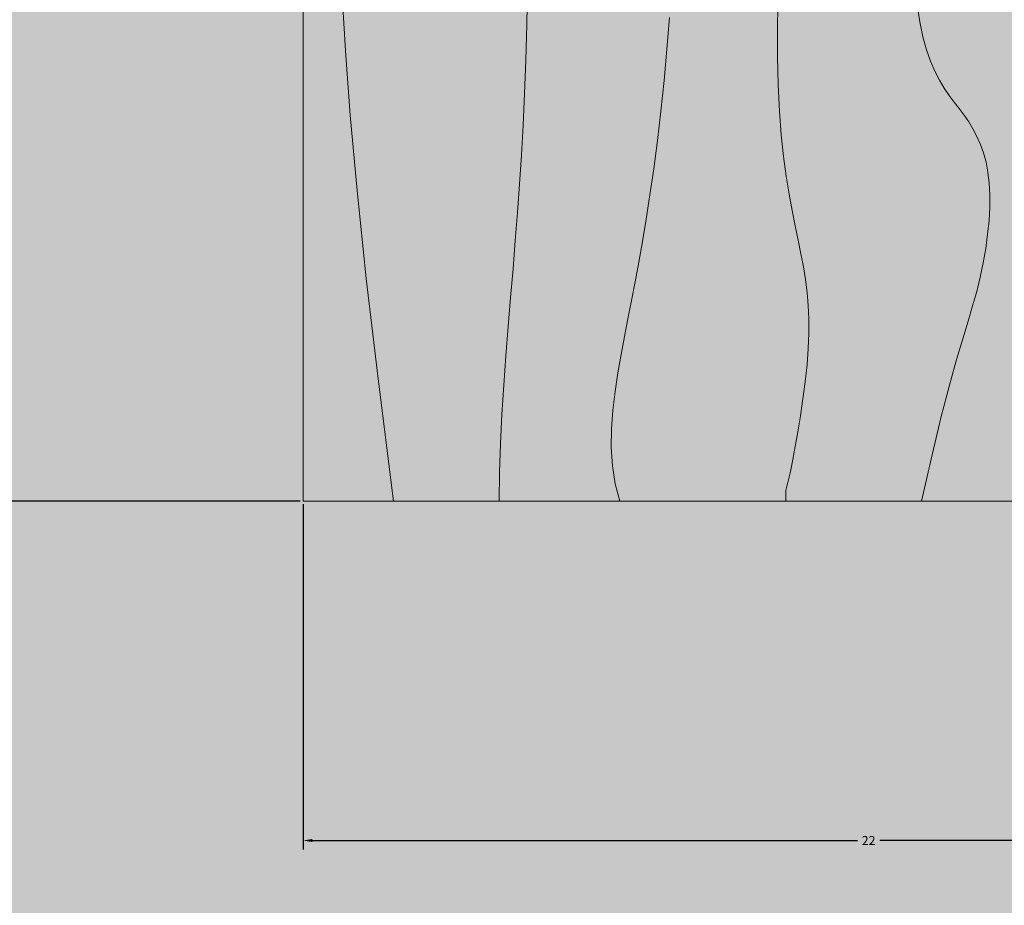
# Model space of a CAD drawing. Units: inches. Extents: x 3024 to 3952, y 1308 to 1863.
# Tile 14 of 29: x 3391.52 to 3411.08, y 1488.75 to 1506.34. Entities that reach past the tile are written whole.
import ezdxf

# ---------------------------------------------------------------- set-up
doc = ezdxf.new("R2010")
doc.units = ezdxf.units.IN
for name, color, linetype, lineweight in [('A-ANNO-DIMS', 2, 'Continuous', 18), ('A-FLOR-TILE-PATT', 7, 'Continuous', 13), ('A-FURN', 8, 'Continuous', 18), ('A-FURN-PATT', 9, 'Continuous', 13)]:
    doc.layers.add(name, color=color, linetype=linetype, lineweight=lineweight)
doc.layers.add('A-FLOR-PATT', color=254, linetype='Continuous', lineweight=13, true_color=0xfeeab9)
doc.styles.get("Standard").update_dxf_attribs({"font": 'arial.ttf'})
doc.dimstyles.get("Standard").update_dxf_attribs({"dimtxt": 0.18, "dimasz": 0.18, "dimexe": 0.18, "dimexo": 0.0625, "dimgap": 0.09, "dimtad": 0, "dimtih": 1, "dimtoh": 1, "dimdec": 4, "dimzin": 0, "dimdsep": 46, "dimtxsty": 'Standard', "dimcen": 0.09, "dimadec": 0, "dimazin": 0, "dimtfac": 1, "dimtdec": 4, "dimtofl": 0, "dimtmove": 0, "dimatfit": 3, "dimfxl": 1, "dimtolj": 1, "dimtzin": 0, "dimarcsym": 0})

# ---------------------------------------------------------------- blocks, each defined once
blk = doc.blocks.new('Table - Rectangular Woodgrain 60 x 30 in.')
for p, q in [((60, -30), (60, 0)), ((0, -30), (60, -30))]:
    blk.add_line(p, q)
for points in [[(46.8439, -13.7104), (47.2906, -13.6417), (47.6858, -13.5604), (48.0333, -13.4667), (48.3375, -13.3608), (48.6042, -13.2448), (48.8396, -13.121), (49.05, -12.9917), (49.2417, -12.8593), (49.4208, -12.7261), (49.5937, -12.5944), (49.7667, -12.4667), (49.9452, -12.3451), (50.1323, -12.2313), (50.3303, -12.1268), (50.5416, -12.0333), (50.7686, -11.9524), (51.0135, -11.8854), (51.2788, -11.8341), (51.5666, -11.8), (51.8785, -11.7843), (52.2116, -11.7865), (52.562, -11.8059), (52.926, -11.8417), (53.2998, -11.8931), (53.6795, -11.9594), (54.0614, -12.0397), (54.4416, -12.1333), (54.8223, -12.2401), (55.2293, -12.3625), (55.6942, -12.5037), (56.2489, -12.6667), (56.9251, -12.8547), (57.7545, -13.0708), (58.7689, -13.3182), (60, -13.6)], [(46.4858, -17.4012), (47.3802, -17.4156), (48.2074, -17.416), (48.9667, -17.4), (49.6583, -17.3662), (50.2872, -17.3167), (50.8595, -17.2547), (51.3812, -17.1833), (51.8584, -17.1057), (52.2971, -17.025), (52.7034, -16.9443), (53.0833, -16.8667), (53.443, -16.7951), (53.789, -16.7313), (54.128, -16.6768), (54.4666, -16.6334), (54.8115, -16.6024), (55.1693, -16.5854), (55.5465, -16.5841), (55.95, -16.6), (56.3828, -16.6337), (56.8346, -16.6823), (57.2915, -16.7418), (57.7396, -16.8084), (58.165, -16.878), (58.5539, -16.9469), (58.8924, -17.0111), (59.1666, -17.0667), (59.3679, -17.1107), (59.5078, -17.1438), (59.6032, -17.1675), (59.6708, -17.1833), (59.7275, -17.193), (59.7901, -17.1979), (59.8753, -17.1998), (60, -17.2)], [(47.1747, -20.2844), (48.0163, -20.3488), (48.8479, -20.425), (49.66, -20.5106), (50.4429, -20.6031), (51.1872, -20.7004), (51.8833, -20.8), (52.5246, -20.8999), (53.1166, -20.9995), (53.6681, -21.0983), (54.1875, -21.1958), (54.6834, -21.2919), (55.1646, -21.3859), (55.6394, -21.4777), (56.1167, -21.5667), (56.6028, -21.6515), (57.0961, -21.7266), (57.5929, -21.7852), (58.0896, -21.8208), (58.5823, -21.8268), (59.0674, -21.7964), (59.5412, -21.723), (60, -21.6)], [(46.3557, -24.0451), (47.3667, -24.0667), (48.309, -24.0947), (49.1928, -24.1287), (50.0284, -24.168), (50.826, -24.2125), (51.5959, -24.2617), (52.3483, -24.3151), (53.0935, -24.3725), (53.8417, -24.4334), (54.6009, -24.497), (55.3699, -24.561), (56.1454, -24.6226), (56.9239, -24.6792), (57.7021, -24.7279), (58.4764, -24.7662), (59.2435, -24.7911), (60, -24.8)], [(46.5843, -28.9641), (48.0579, -28.8816), (49.7666, -28.7542), (51.7629, -28.5721), (54.0989, -28.3255), (56.8272, -28.0048), (60, -27.6)]]:
    blk.add_lwpolyline(points)
blk = doc.blocks.new('*D32')
at = {"layer": 'A-ANNO-DIMS', "color": 0, "lineweight": -2, "transparency": 16777216}
for p, q in [((3397.088, 1541.715), (3390.23, 1541.715)), ((3390.41, 1541.535), (3390.41, 1519.428)), ((3390.41, 1496.958), (3390.41, 1519.065)), ((3397.088, 1496.778), (3390.23, 1496.778))]:
    blk.add_line(p, q, dxfattribs=at)
at = {"layer": 'A-ANNO-DIMS', "color": 0, "transparency": 16777216}
for points in [[(3390.38, 1541.535), (3390.44, 1541.535), (3390.41, 1541.715)], [(3390.38, 1496.958), (3390.44, 1496.958), (3390.41, 1496.778)]]:
    blk.add_solid(points, dxfattribs=at)
at = {"layer": 'Defpoints', "color": 0, "transparency": 16777216}
for p in [(3397.15, 1541.715), (3390.41, 1496.778), (3397.15, 1496.778)]:
    blk.add_point(p, dxfattribs=at)
at = {"layer": 'A-ANNO-DIMS', "color": 0, "transparency": 16777216, "insert": (3390.41, 1519.246), "char_height": 0.18, "attachment_point": 5}
blk.add_mtext('\\A1;TABLE 45', dxfattribs=at)
blk = doc.blocks.new('*D33')
at = {"layer": 'A-ANNO-DIMS', "color": 0, "lineweight": -2, "transparency": 16777216}
for p, q in [((3397.15, 1496.716), (3397.15, 1489.858)), ((3419.618, 1496.716), (3419.618, 1489.858)), ((3397.33, 1490.038), (3408.165, 1490.038)), ((3419.438, 1490.038), (3408.604, 1490.038))]:
    blk.add_line(p, q, dxfattribs=at)
at = {"layer": 'A-ANNO-DIMS', "color": 0, "transparency": 16777216}
for points in [[(3397.33, 1490.068), (3397.33, 1490.008), (3397.15, 1490.038)], [(3419.438, 1490.068), (3419.438, 1490.008), (3419.618, 1490.038)]]:
    blk.add_solid(points, dxfattribs=at)
at = {"layer": 'Defpoints', "color": 0, "transparency": 16777216}
for p in [(3397.15, 1496.778), (3419.618, 1496.778), (3419.618, 1490.038)]:
    blk.add_point(p, dxfattribs=at)
at = {"layer": 'A-ANNO-DIMS', "color": 0, "transparency": 16777216, "insert": (3408.384, 1490.038), "char_height": 0.18, "attachment_point": 5}
blk.add_mtext('\\A1;22', dxfattribs=at)

msp = doc.modelspace()

# ---------------------------------------------------------------- hatches: boundary and pattern name
at = {"layer": 'A-FLOR-PATT', "transparency": 33554528}
h = msp.add_hatch(color=256, dxfattribs=at)
h.dxf.hatch_style = 1
h.paths.add_polyline_path([(3460.764, 1688.6064), (3412.764, 1688.6064), (3412.764, 1694.6064), (3460.764, 1694.6064), (3460.764, 1778.6064), (3406.764, 1778.6064), (3406.764, 1759.9514), (3318.2981, 1759.9514), (3318.2981, 1658.6064), (3322.5356, 1658.6064), (3322.5356, 1652.6064), (3292.764, 1652.6064), (3292.764, 1778.6064), (3106.764, 1778.6064), (3106.764, 1628.6064), (3172.764, 1628.6064), (3172.764, 1532.6064), (3166.764, 1532.6064), (3166.764, 1628.6064), (3106.764, 1628.6064), (3106.764, 1356.8452), (3202.812, 1356.8452), (3202.812, 1354.2534), (3202.812, 1353.8388), (3202.812, 1351.1212), (3202.812, 1347.8452), (3277.764, 1347.8452), (3277.764, 1353.8452), (3277.764, 1356.8452), (3277.764, 1442.6064), (3460.764, 1442.6064)])
h.paths.add_polyline_path([(3216.238, 1527.2064), (3216.238, 1491.2064), (3214.663, 1491.2064), (3214.663, 1491.2409, -0.3966224), (3180.243, 1526.6064), (3163.0285, 1526.6064), (3163.0285, 1531.1064), (3161.716, 1531.1064), (3161.716, 1561.1064), (3163.0285, 1561.1064), (3163.0285, 1531.1064), (3163.0285, 1526.6064), (3180.243, 1526.6064, 0.3966224), (3214.663, 1491.2409), (3214.663, 1527.2064)], flags=16)
h.paths.add_polyline_path([(3227.364, 1649.8972), (3191.364, 1649.8972), (3191.364, 1651.4722), (3227.364, 1651.4722)], flags=16)
h.paths.add_polyline_path([(3323.1172, 1606.7362), (3323.8545, 1606.8514), (3323.8545, 1594.8241), (3323.1172, 1594.9393)], flags=16)
h.paths.add_polyline_path([(3324.2232, 1606.909), (3330.1216, 1607.8307), (3330.1216, 1614.1093), (3339.3495, 1614.1093), (3340.2711, 1620.0078), (3352.4136, 1620.0078), (3353.3353, 1614.1093), (3359.9941, 1614.1093), (3360.9157, 1620.0078), (3373.0582, 1620.0078), (3373.9799, 1614.1093), (3383.2077, 1614.1093), (3383.2077, 1607.8307), (3389.1062, 1606.909), (3389.1062, 1594.7665), (3383.2077, 1593.8449), (3383.2077, 1587.5663), (3373.9799, 1587.5663), (3373.0583, 1581.6678), (3360.9157, 1581.6678), (3359.9941, 1587.5663), (3353.3353, 1587.5663), (3352.4136, 1581.6678), (3340.2711, 1581.6678), (3339.3495, 1587.5663), (3330.1216, 1587.5663), (3330.1216, 1593.8449), (3324.2232, 1594.7665)], flags=16)
h.paths.add_polyline_path([(3236.1584, 1693.1064), (3236.1584, 1723.1064), (3237.4709, 1723.1064), (3237.4709, 1693.1064)], flags=16)
h.paths.add_polyline_path([(3373.2158, 1600.6847), (3373.7965, 1600.7303), (3374.3268, 1600.7874), (3374.8132, 1600.8531), (3375.2621, 1600.9247), (3375.6801, 1600.9991), (3376.0736, 1601.0735), (3376.6855, 1601.19), (3377.366, 1601.3023), (3378.0667, 1601.3814), (3378.8026, 1601.4123), (3379.5865, 1601.3839), (3380.4537, 1601.2948), (3381.301, 1601.1717), (3382.0317, 1601.0433), (3382.4398, 1600.9607), (3382.6252, 1600.9201), (3382.919, 1600.8507), (3382.9044, 1600.8531), (3382.842, 1600.8678), (3382.7541, 1600.8896), (3382.6252, 1600.9201), (3382.4398, 1600.9607), (3382.1868, 1601.0119), (3381.8738, 1601.0711), (3381.5125, 1601.1346), (3381.1149, 1601.1988), (3380.6928, 1601.2601), (3380.2581, 1601.3149), (3379.8226, 1601.3597), (3379.3984, 1601.3908), (3378.9944, 1601.4054), (3378.6092, 1601.4042), (3378.2384, 1601.3886), (3377.8777, 1601.36), (3377.5227, 1601.32), (3377.1691, 1601.2698), (3376.8127, 1601.211), (3376.4491, 1601.145), (3376.0736, 1601.0735), (3375.4177, 1600.9494), (3374.5542, 1600.8119), (3373.5044, 1600.6988)], flags=0)
h.paths.add_polyline_path([(3380.0253, 1596.7351), (3380.499, 1596.6659), (3380.9706, 1596.6119), (3381.4375, 1596.5791), (3381.8971, 1596.5736), (3382.5886, 1596.6167), (3382.7848, 1596.6692), (3382.1465, 1596.5706), (3381.236, 1596.5815), (3380.3199, 1596.6865)], flags=0)
h.paths.add_polyline_path([(3369.6414, 1603.9617), (3370.1589, 1604.0021), (3370.6218, 1604.0539), (3371.0335, 1604.1173), (3371.3978, 1604.1921), (3371.7181, 1604.2785), (3371.9984, 1604.3761), (3372.2441, 1604.483), (3372.4611, 1604.5972), (3372.655, 1604.7163), (3372.8317, 1604.8384), (3372.9968, 1604.9611), (3373.3703, 1605.2455), (3373.8426, 1605.5328), (3374.4624, 1605.7539), (3375.1058, 1605.8302), (3375.7221, 1605.8261), (3376.4109, 1605.76), (3377.1534, 1605.6376), (3377.8945, 1605.473), (3378.1382, 1605.409), (3377.7394, 1605.5074), (3377.3509, 1605.5937), (3376.9704, 1605.6677), (3376.5999, 1605.7288), (3376.2417, 1605.7762), (3375.8979, 1605.8092), (3375.5707, 1605.8271), (3375.2621, 1605.8291), (3374.9745, 1605.8146), (3374.7092, 1605.7832), (3374.4647, 1605.7359), (3374.239, 1605.6742), (3374.0298, 1605.5996), (3373.835, 1605.5134), (3373.6525, 1605.4171), (3373.4801, 1605.3123), (3373.3156, 1605.2002), (3373.1562, 1605.0825), (3372.7603, 1604.781), (3372.236, 1604.4588), (3371.5738, 1604.2283), (3370.8493, 1604.0794), (3369.9262, 1603.976)], flags=0)
h.paths.add_polyline_path([(3366.7533, 1606.5832), (3367.1713, 1606.5519), (3367.5378, 1606.5374), (3367.8568, 1606.5394), (3368.1325, 1606.5573), (3368.3694, 1606.5903), (3368.5717, 1606.6377), (3368.7438, 1606.6988), (3368.89, 1606.7728), (3369.0146, 1606.8591), (3369.121, 1606.9568), (3369.2094, 1607.0646), (3369.2792, 1607.181), (3369.3295, 1607.3046), (3369.3596, 1607.4339), (3369.3688, 1607.5676), (3369.3565, 1607.7042), (3369.3218, 1607.8422), (3369.2649, 1607.9804), (3369.1893, 1608.1187), (3369.0993, 1608.2569), (3368.9992, 1608.3952), (3368.8934, 1608.5334), (3368.7861, 1608.6717), (3368.6817, 1608.8099), (3368.4212, 1609.1804), (3368.2685, 1609.7106), (3368.4883, 1610.1814), (3369.0537, 1610.4604), (3369.6717, 1610.5097), (3370.2812, 1610.3612), (3370.4805, 1610.2968), (3370.1882, 1610.3839), (3369.9284, 1610.4472), (3369.6905, 1610.4842), (3369.4662, 1610.4933), (3369.2555, 1610.4765), (3369.0608, 1610.4367), (3368.884, 1610.3767), (3368.7274, 1610.2994), (3368.5931, 1610.2077), (3368.4833, 1610.1045), (3368.4002, 1609.9927), (3368.3451, 1609.8747), (3368.3166, 1609.7517), (3368.3127, 1609.6244), (3368.331, 1609.4935), (3368.3696, 1609.3597), (3368.4261, 1609.2237), (3368.4985, 1609.0863), (3368.5845, 1608.9482), (3368.6817, 1608.8099), (3368.7861, 1608.6717), (3368.8934, 1608.5334), (3368.9992, 1608.3952), (3369.0993, 1608.2569), (3369.3398, 1607.8876), (3369.3941, 1607.2896), (3368.9774, 1606.7817), (3368.3928, 1606.5742), (3367.7162, 1606.5303), (3367.0044, 1606.5585)], flags=0)
h.paths.add_polyline_path([(3362.1859, 1610.2589), (3362.5478, 1610.2845), (3362.8348, 1610.3275), (3363.0585, 1610.3863), (3363.2303, 1610.4595), (3363.3619, 1610.5457), (3363.463, 1610.6432), (3363.5376, 1610.7502), (3363.5876, 1610.8643), (3363.6153, 1610.9834), (3363.6229, 1611.1055), (3363.6125, 1611.2283), (3363.5861, 1611.3496), (3363.5462, 1611.4673), (3363.4949, 1611.5797), (3363.4358, 1611.6871), (3363.3723, 1611.7902), (3363.3081, 1611.8897), (3363.2468, 1611.9863), (3363.192, 1612.0808), (3363.0258, 1612.4261), (3363.3371, 1612.8672), (3363.9008, 1612.9782), (3364.4822, 1612.9641), (3365.1098, 1612.9074), (3365.328, 1612.8805), (3364.9615, 1612.9208), (3364.6426, 1612.9496), (3364.3668, 1612.9669), (3364.1299, 1612.9726), (3363.9276, 1612.9669), (3363.7555, 1612.9496), (3363.6093, 1612.9208), (3363.4848, 1612.8805), (3363.3782, 1612.8289), (3363.2889, 1612.7672), (3363.2169, 1612.6969), (3363.1622, 1612.6193), (3363.1247, 1612.5361), (3363.1046, 1612.4484), (3363.1017, 1612.358), (3363.1161, 1612.266), (3363.1472, 1612.1738), (3363.192, 1612.0808), (3363.2468, 1611.9863), (3363.3081, 1611.8897), (3363.3723, 1611.7902), (3363.4358, 1611.6871), (3363.6363, 1611.323), (3363.5979, 1610.7003), (3363.0863, 1610.3651), (3362.3983, 1610.2622)], flags=0)
h.paths.add_polyline_path([(3352.356, 1581.2991), (3352.2408, 1580.5618), (3340.4439, 1580.5618), (3340.3287, 1581.2991)], flags=16)
h.paths.add_polyline_path([(3340.4439, 1621.1137), (3352.2408, 1621.1137), (3352.356, 1620.3764), (3340.3287, 1620.3764)], flags=16)
h.paths.add_polyline_path([(3278.4282, 1504.7424), (3290.3831, 1504.7424), (3290.3831, 1502.7499), (3291.0473, 1502.7499), (3291.0473, 1494.7799), (3290.3831, 1494.7799), (3290.3831, 1494.1158), (3291.0473, 1494.1158), (3291.0473, 1486.1458), (3290.3831, 1486.1458), (3290.3831, 1484.1533), (3291.0473, 1484.1533), (3291.0473, 1483.4892, -0.0909091), (3291.0473, 1468.8776), (3291.0473, 1468.2135), (3290.3831, 1468.2135), (3290.3831, 1464.8926), (3278.4282, 1464.8926), (3278.4282, 1472.8626), (3277.764, 1473.5268), (3277.764, 1478.84), (3278.4282, 1479.5042)], flags=16)
h.paths.add_polyline_path([(3278.7603, 1504.4103), (3290.051, 1504.4103), (3290.051, 1465.2247), (3278.7603, 1465.2247)], flags=0)
h.paths.add_polyline_path([(3123.904, 1600.7821), (3117.9039, 1602.7821), (3117.9039, 1599.7821), (3119.4039, 1599.7821), (3119.4039, 1596.7821), (3118.4039, 1596.7821), (3118.4039, 1598.7821), (3117.9039, 1598.7821), (3117.9039, 1596.2821), (3109.9039, 1596.2821), (3109.9039, 1617.2821), (3117.9039, 1617.2821), (3117.9039, 1610.7821), (3123.9038, 1612.7821, -0.7025712), (3137.9039, 1606.7822, -0.7025621)], flags=16)
h.paths.add_polyline_path([(3123.9039, 1602.7822), (3123.9039, 1610.7822, -0.7345333), (3136.9039, 1606.7822, -0.7345297)], flags=0)
h.paths.add_polyline_path([(3177.972, 1689.6473), (3109.2405, 1689.6473), (3109.2405, 1741.1959), (3177.972, 1741.1959)], flags=16)
h.paths.add_polyline_path([(3373.0006, 1581.2991), (3372.8854, 1580.5618), (3361.0885, 1580.5618), (3360.9733, 1581.2991)], flags=16)
h.paths.add_polyline_path([(3361.0885, 1621.1137), (3372.8854, 1621.1137), (3373.0006, 1620.3764), (3360.9733, 1620.3764)], flags=16)
h.paths.add_polyline_path([(3116.9039, 1598.2821, -0.4142136), (3116.1539, 1597.2821), (3111.9039, 1597.2821, -0.4142136), (3110.9039, 1598.0321), (3110.9039, 1615.2821, -0.4142136), (3111.6539, 1616.2821), (3115.9039, 1616.2821, -0.4142136), (3116.9039, 1615.5321)], flags=0)
h.paths.add_polyline_path([(3121.6122, 1728.1369), (3121.6122, 1696.5205), (3110.2715, 1696.5205), (3110.2715, 1714.3906), (3121.6122, 1714.3906), (3121.6122, 1716.4526), (3110.2715, 1716.4526), (3110.2715, 1734.3228), (3123.3304, 1734.3228), (3123.3304, 1729.8552), (3134.6711, 1741.1959), (3134.6711, 1728.1369)], flags=0)
h.paths.add_polyline_path([(3389.4748, 1606.8514), (3390.2122, 1606.7362), (3390.2122, 1594.9393), (3389.4748, 1594.8241)], flags=16)
h.paths.add_polyline_path([(3257.6842, 1762.8281), (3259.6842, 1768.8281), (3256.6842, 1768.8281), (3256.6842, 1767.3281), (3253.6842, 1767.3281), (3253.6842, 1768.3281), (3255.6842, 1768.3281), (3255.6842, 1768.8281), (3253.1842, 1768.8281), (3253.1842, 1776.8281), (3274.1842, 1776.8281), (3274.1842, 1768.8281), (3267.6842, 1768.8281), (3269.6842, 1762.8282, -0.7025712), (3263.6843, 1748.8282, -0.7025621)], flags=16)
h.paths.add_polyline_path([(3259.6842, 1762.8281), (3267.6843, 1762.8281, -0.7345333), (3263.6842, 1749.8282, -0.7345297)], flags=0)
h.paths.add_polyline_path([(3411.264, 1715.6064), (3411.264, 1716.9189), (3441.264, 1716.9189), (3441.264, 1715.6064)], flags=16)
h.paths.add_polyline_path([(3178.3806, 1449.1876), (3178.3806, 1397.639), (3109.6491, 1397.639), (3109.6491, 1449.1876)], flags=16)
h.paths.add_polyline_path([(3397.1501, 1541.7146), (3419.6183, 1541.7146), (3419.6183, 1496.7783), (3397.1501, 1496.7783)], flags=16)
h.paths.add_polyline_path([(3254.1842, 1770.5781), (3254.1842, 1774.8281, -0.4142136), (3254.9342, 1775.8281), (3272.1842, 1775.8281, -0.4142136), (3273.1842, 1775.0781), (3273.1842, 1770.8281, -0.4142136), (3272.4342, 1769.8281), (3255.1842, 1769.8281, -0.4142136)], flags=0)
h.paths.add_polyline_path([(3403.672, 1500.7601), (3403.6016, 1500.3997), (3403.5328, 1500.0441), (3403.4662, 1499.6867), (3403.4027, 1499.3226), (3403.3464, 1498.9532), (3403.3025, 1498.5811), (3403.2759, 1498.2091), (3403.2714, 1497.8401), (3403.3064, 1497.2813), (3403.3491, 1497.1219), (3403.2689, 1497.6395), (3403.2778, 1498.3719), (3403.3635, 1499.0984), (3403.4889, 1499.8168), (3403.6016, 1500.3997), (3403.672, 1500.7601), (3403.744, 1501.1315), (3403.817, 1501.5205), (3403.891, 1501.9336), (3403.9656, 1502.3769), (3404.0404, 1502.8572), (3404.115, 1503.3786), (3404.2264, 1504.2311), (3404.2571, 1504.5223), (3404.1552, 1503.6598), (3404.0063, 1502.6193), (3403.8604, 1501.7518), (3403.744, 1501.1315)], flags=0)
h.paths.add_polyline_path([(3406.5868, 1505.0416), (3406.6121, 1504.5236), (3406.6492, 1504.0526), (3406.6956, 1503.624), (3406.7491, 1503.2333), (3406.8072, 1502.8759), (3406.8676, 1502.5473), (3406.9281, 1502.243), (3407.0268, 1501.7597), (3407.1416, 1501.1368), (3407.2087, 1500.3904), (3407.1804, 1499.6703), (3407.1078, 1498.9956), (3407.0074, 1498.3199), (3406.8809, 1497.6059), (3406.7403, 1496.9627), (3406.7418, 1496.9824), (3406.7491, 1497.0249), (3406.8229, 1497.3409), (3406.8364, 1497.4025), (3406.878, 1497.6078), (3406.9261, 1497.8614), (3406.9777, 1498.1526), (3407.0298, 1498.4712), (3407.0797, 1498.8068), (3407.1243, 1499.149), (3407.1607, 1499.4874), (3407.1859, 1499.8115), (3407.1978, 1500.1137), (3407.1969, 1500.3962), (3407.1841, 1500.6642), (3407.1609, 1500.9225), (3407.1284, 1501.1761), (3407.0876, 1501.43), (3407.0398, 1501.6891), (3406.9862, 1501.9585), (3406.8832, 1502.4628), (3406.7712, 1503.0713), (3406.6657, 1503.8424), (3406.5924, 1504.7735)], flags=0)
h.paths.add_polyline_path([(3409.2517, 1507.8962), (3409.2752, 1507.4282), (3409.3079, 1507.0076), (3409.3501, 1506.6314), (3409.4015, 1506.2969), (3409.4624, 1506.0009), (3409.5326, 1505.7406), (3409.6119, 1505.5128), (3409.6988, 1505.3131), (3409.7915, 1505.1368), (3409.8883, 1504.9792), (3409.9875, 1504.8356), (3410.0872, 1504.7015), (3410.1859, 1504.572), (3410.4508, 1504.2132), (3410.7205, 1503.6035), (3410.8059, 1502.8824), (3410.7619, 1502.0875), (3410.6122, 1501.2299), (3410.4402, 1500.6169), (3410.2538, 1500.0031), (3410.0536, 1499.3219), (3409.9909, 1499.0812), (3410.1761, 1499.7472), (3410.3596, 1500.3513), (3410.4512, 1500.6561), (3410.5312, 1500.9412), (3410.6013, 1501.226), (3410.6614, 1501.512), (3410.7111, 1501.7964), (3410.7496, 1502.0763), (3410.7764, 1502.3489), (3410.7909, 1502.6114), (3410.7926, 1502.8608), (3410.7808, 1503.0944), (3410.7553, 1503.31), (3410.7169, 1503.5087), (3410.6667, 1503.6921), (3410.6061, 1503.8621), (3410.5361, 1504.0203), (3410.4578, 1504.1686), (3410.3726, 1504.3088), (3410.2815, 1504.4424), (3410.1859, 1504.572), (3410.0872, 1504.7015), (3409.859, 1505.0083), (3409.5943, 1505.5117), (3409.4266, 1506.1336), (3409.324, 1506.8011), (3409.2586, 1507.6407)], flags=0)
h.paths.add_polyline_path([(3411.4914, 1510.5878), (3411.4432, 1510.1586), (3411.4054, 1509.775), (3411.38, 1509.4354), (3411.3681, 1509.1376), (3411.3698, 1508.8784), (3411.3843, 1508.6542), (3411.4112, 1508.4618), (3411.4497, 1508.2974), (3411.4994, 1508.1575), (3411.5595, 1508.0388), (3411.6296, 1507.9375), (3411.7097, 1507.851), (3411.802, 1507.7792), (3411.9096, 1507.7225), (3412.0353, 1507.6817), (3412.1821, 1507.6572), (3412.3528, 1507.6496), (3412.5505, 1507.6597), (3412.778, 1507.6879), (3413.0364, 1507.7341), (3413.3194, 1507.7955), (3413.6188, 1507.8687), (3413.9264, 1507.95), (3414.234, 1508.036), (3414.5333, 1508.1232), (3414.8163, 1508.208), (3415.0747, 1508.287), (3415.3023, 1508.3569), (3415.5007, 1508.4158), (3415.6733, 1508.4617), (3416.1158, 1508.5538), (3416.512, 1508.2591), (3416.716, 1507.6581), (3416.61, 1507.0003), (3416.3052, 1506.3411), (3415.8928, 1505.618), (3415.7339, 1505.3633), (3415.9914, 1505.791), (3416.201, 1506.1583), (3416.3666, 1506.4739), (3416.4925, 1506.7462), (3416.5828, 1506.9838), (3416.6413, 1507.1949), (3416.6725, 1507.3883), (3416.6799, 1507.5705), (3416.6662, 1507.7417), (3416.6339, 1507.9), (3416.5851, 1508.0436), (3416.5223, 1508.1709), (3416.4478, 1508.28), (3416.3639, 1508.3692), (3416.273, 1508.4368), (3416.1765, 1508.4815), (3416.0718, 1508.5047), (3415.9553, 1508.5079), (3415.8237, 1508.493), (3415.6733, 1508.4617), (3415.5007, 1508.4158), (3415.3327, 1508.3659), (3414.6495, 1508.157), (3414.0606, 1507.9855), (3413.4456, 1507.8229), (3412.8838, 1507.701), (3412.5505, 1507.6597), (3412.0748, 1507.6354), (3411.595, 1507.8883), (3411.398, 1508.4429), (3411.3624, 1508.9927), (3411.3854, 1509.5711), (3411.4578, 1510.3071)], flags=0)
h.paths.add_polyline_path([(3135.0797, 1449.1876), (3135.0797, 1436.1286), (3122.0208, 1436.1286), (3122.0208, 1404.5122), (3110.6801, 1404.5122), (3110.6801, 1422.3823), (3122.0208, 1422.3823), (3122.0208, 1424.4443), (3110.6801, 1424.4443), (3110.6801, 1442.3145), (3123.739, 1442.3145), (3123.739, 1437.8469)], flags=0)
h.paths.add_polyline_path([(3416.4944, 1514.2949), (3416.4837, 1513.8511), (3416.4893, 1513.4867), (3416.5102, 1513.1926), (3416.5451, 1512.9593), (3416.5929, 1512.7775), (3416.6524, 1512.6379), (3416.7224, 1512.531), (3416.8017, 1512.4488), (3416.8886, 1512.3882), (3416.9813, 1512.3476), (3417.0781, 1512.3251), (3417.1773, 1512.3189), (3417.277, 1512.3274), (3417.3757, 1512.3488), (3417.4713, 1512.3813), (3417.5627, 1512.4229), (3417.65, 1512.471), (3417.7338, 1512.5225), (3417.8146, 1512.5747), (3417.8931, 1512.6245), (3417.9699, 1512.6691), (3418.2968, 1512.8265), (3418.6505, 1512.4645), (3418.7037, 1511.9342), (3418.6693, 1511.3839), (3418.6076, 1510.8228), (3418.5777, 1510.5927), (3418.6197, 1510.9333), (3418.6525, 1511.2311), (3418.6759, 1511.4903), (3418.6899, 1511.7144), (3418.6946, 1511.9069), (3418.6899, 1512.0713), (3418.6759, 1512.2112), (3418.6525, 1512.33), (3418.6197, 1512.4311), (3418.5778, 1512.5177), (3418.5276, 1512.5903), (3418.4705, 1512.6488), (3418.4075, 1512.6933), (3418.3399, 1512.7237), (3418.2686, 1512.7401), (3418.1951, 1512.7424), (3418.1204, 1512.7307), (3418.0455, 1512.7055), (3417.9792, 1512.6736), (3417.65, 1512.471), (3417.5627, 1512.4229), (3417.4713, 1512.3813), (3417.3757, 1512.3488), (3417.277, 1512.3274), (3416.878, 1512.2936), (3416.5757, 1512.7549), (3416.492, 1513.3145), (3416.4808, 1514.0384)], flags=0)
h.paths.add_polyline_path([(3392.8223, 1481.9454), (3396.7707, 1481.9454), (3396.7707, 1480.9201), (3428.3585, 1480.9201), (3428.3585, 1481.9454), (3432.3069, 1481.9454), (3432.3069, 1464.8354, -0.266667), (3392.8223, 1464.8354)], flags=16)
h.paths.add_polyline_path([(3431.203, 1547.5428), (3450.8613, 1547.5428, -0.1904762), (3450.8614, 1484.031), (3431.203, 1484.031), (3431.203, 1488.5675), (3432.3809, 1488.5675), (3432.3809, 1543.0062), (3431.203, 1543.0062)], flags=16)
h.paths.add_polyline_path([(3451.9233, 1524.86, -0.0496282), (3451.9233, 1506.7138), (3446.7921, 1506.7138), (3446.7921, 1524.86)], flags=0)
h.paths.add_polyline_path([(3460.764, 1436.6064), (3277.764, 1436.6064), (3277.764, 1356.8452), (3277.764, 1353.8452), (3460.764, 1353.8452)], flags=17)
h.paths.add_polyline_path([(3121.3033, 1577.378), (3153.693, 1577.378), (3153.693, 1586.6752), (3121.3033, 1586.6752)], flags=24)
h.paths.add_polyline_path([(3164.1457, 1464.1276), (3210.4801, 1464.1276), (3210.4801, 1473.4247), (3164.1457, 1473.4247)], flags=24)
h.paths.add_polyline_path([(3343.1909, 1505.8863), (3373.7236, 1505.8863), (3373.7236, 1515.1773), (3343.1909, 1515.1773)], flags=24)
h.paths.add_polyline_path([(3337.6353, 1564.2926), (3370.0189, 1564.2926), (3370.0189, 1573.5836), (3337.6353, 1573.5836)], flags=24)
h.paths.add_polyline_path([(3419.204, 1753.8578), (3453.3997, 1753.8578), (3453.3997, 1762.9956), (3419.204, 1762.9956)], flags=24)
h.paths.add_polyline_path([(3341.2523, 1701.0246), (3381.0761, 1701.0246), (3381.0761, 1710.3156), (3341.2523, 1710.3156)], flags=24)
h.paths.add_polyline_path([(3245.8895, 1726.2997), (3278.2793, 1726.2997), (3278.2793, 1735.5968), (3245.8895, 1735.5968)], flags=24)
h.paths.add_polyline_path([(3128.8045, 1668.6736), (3175.1389, 1668.6736), (3175.1389, 1677.9707), (3128.8045, 1677.9707)], flags=24)
h.paths.add_polyline_path([(3345.9997, 1396.0062), (3389.09, 1396.0062), (3389.09, 1405.3033), (3345.9997, 1405.3033)], flags=24)
at = {"layer": 'A-FLOR-TILE-PATT', "transparency": 33554569}
h = msp.add_hatch(dxfattribs=at)
h.set_pattern_fill('ANGLE', color=256, scale=2)
h.set_pattern_definition([(0, (0, 0), (0, 13.97), [10.16, -3.81]), (90, (0, 0), (-13.97, 9e-16), [10.16, -3.81])])
h.paths.add_polyline_path([(3292.764, 1778.6064), (3232.764, 1778.6064), (3232.764, 1694.6064), (3236.1584, 1694.6064), (3236.1584, 1723.1064), (3237.4709, 1723.1064), (3237.4709, 1723.0777, -0.3870039), (3266.1209, 1694.6064), (3292.764, 1694.6064)])
h.paths.add_polyline_path([(3263.6843, 1748.8282, -0.7025621), (3257.6842, 1762.8281), (3259.6842, 1768.8281), (3256.6842, 1768.8281), (3256.6842, 1767.3281), (3253.6842, 1767.3281), (3253.6842, 1768.3281), (3255.6842, 1768.3281), (3255.6842, 1768.8281), (3253.1842, 1768.8281), (3253.1842, 1776.8281), (3274.1842, 1776.8281), (3274.1842, 1768.8281), (3267.6842, 1768.8281), (3269.6842, 1762.8282, -0.7025712)], flags=16)
h.paths.add_polyline_path([(3263.6842, 1749.8282, -0.7345297), (3259.6842, 1762.8281), (3267.6843, 1762.8281, -0.7345333)], flags=0)
h.paths.add_polyline_path([(3255.1842, 1769.8281, -0.4142136), (3254.1842, 1770.5781), (3254.1842, 1774.8281, -0.4142136), (3254.9342, 1775.8281), (3272.1842, 1775.8281, -0.4142136), (3273.1842, 1775.0781), (3273.1842, 1770.8281, -0.4142136), (3272.4342, 1769.8281)], flags=0)
h.paths.add_polyline_path([(3460.764, 1436.6064), (3277.764, 1436.6064), (3277.764, 1356.8452), (3277.764, 1353.8452), (3460.764, 1353.8452)])
h.paths.add_polyline_path([(3166.764, 1628.6064), (3106.764, 1628.6064), (3106.764, 1532.6064), (3133.066, 1532.6064, -0.3870039), (3161.716, 1561.0777), (3161.716, 1561.1064), (3163.0285, 1561.1064), (3163.0285, 1532.6064), (3166.764, 1532.6064)])
h.paths.add_polyline_path([(3123.904, 1600.7821), (3117.9039, 1602.7821), (3117.9039, 1599.7821), (3119.4039, 1599.7821), (3119.4039, 1596.7821), (3118.4039, 1596.7821), (3118.4039, 1598.7821), (3117.9039, 1598.7821), (3117.9039, 1596.2821), (3109.9039, 1596.2821), (3109.9039, 1617.2821), (3117.9039, 1617.2821), (3117.9039, 1610.7821), (3123.9038, 1612.7821, -0.7025712), (3137.9039, 1606.7822, -0.7025621)], flags=16)
h.paths.add_polyline_path([(3123.9039, 1602.7822), (3123.9039, 1610.7822, -0.7345333), (3136.9039, 1606.7822, -0.7345297)], flags=0)
h.paths.add_polyline_path([(3116.1539, 1597.2821), (3111.9039, 1597.2821, -0.4142136), (3110.9039, 1598.0321), (3110.9039, 1615.2821, -0.4142136), (3111.6539, 1616.2821), (3115.9039, 1616.2821, -0.4142136), (3116.9039, 1615.5321), (3116.9039, 1598.2821, -0.4142136)], flags=0)
h.paths.add_polyline_path([(3245.8895, 1726.2997), (3278.2793, 1726.2997), (3278.2793, 1735.5968), (3245.8895, 1735.5968)], flags=24)
h.paths.add_polyline_path([(3345.9997, 1396.0062), (3389.09, 1396.0062), (3389.09, 1405.3033), (3345.9997, 1405.3033)], flags=24)
h.paths.add_polyline_path([(3121.3033, 1577.378), (3153.693, 1577.378), (3153.693, 1586.6752), (3121.3033, 1586.6752)], flags=24)
at = {"layer": 'A-FURN-PATT', "transparency": 33554600}
h = msp.add_hatch(color=256, dxfattribs=at)
h.dxf.hatch_style = 1
h.paths.add_polyline_path([(3417.3334, 1524.2182), (3417.4417, 1525.8535), (3417.5429, 1527.6959), (3417.6336, 1529.794), (3417.7102, 1532.1964), (3417.7693, 1534.9516), (3417.8074, 1538.1081), (3417.8209, 1541.7146), (3412.7281, 1541.7146), (3412.8136, 1536.7897), (3412.8505, 1532.7734), (3412.8466, 1529.5424), (3412.8092, 1526.9731), (3412.7461, 1524.942), (3412.6649, 1523.3259), (3412.5731, 1522.0011), (3412.4784, 1520.8443), (3412.3871, 1519.7527), (3412.2998, 1518.707), (3412.216, 1517.7088), (3412.1351, 1516.7594), (3412.0566, 1515.8603), (3411.9799, 1515.013), (3411.9043, 1514.219), (3411.8293, 1513.4797), (3411.7548, 1512.7959), (3411.6819, 1512.1667), (3411.6125, 1511.5901), (3411.5485, 1511.0643), (3411.4914, 1510.5878), (3411.4432, 1510.1586), (3411.4054, 1509.775), (3411.38, 1509.4354), (3411.3681, 1509.1376), (3411.3698, 1508.8784), (3411.3843, 1508.6542), (3411.4112, 1508.4618), (3411.4497, 1508.2974), (3411.4994, 1508.1575), (3411.5595, 1508.0388), (3411.6296, 1507.9375), (3411.7097, 1507.851), (3411.802, 1507.7792), (3411.9096, 1507.7225), (3412.0353, 1507.6817), (3412.1821, 1507.6572), (3412.3528, 1507.6496), (3412.5505, 1507.6597), (3412.778, 1507.6879), (3413.0364, 1507.7341), (3413.3194, 1507.7955), (3413.6188, 1507.8687), (3413.9264, 1507.95), (3414.234, 1508.036), (3414.5333, 1508.1232), (3414.8163, 1508.208), (3415.0747, 1508.287), (3415.4508, 1508.4025), (3415.8572, 1508.5106), (3416.186, 1508.5015), (3416.4107, 1508.3344), (3416.5614, 1508.1136), (3416.6596, 1507.8241), (3416.6872, 1507.4795), (3416.6413, 1507.1949), (3416.5828, 1506.9838), (3416.4925, 1506.7462), (3416.3666, 1506.4739), (3416.201, 1506.1583), (3415.9914, 1505.791), (3415.7339, 1505.3633), (3415.4242, 1504.8669), (3415.0615, 1504.292), (3414.6566, 1503.6241), (3414.2236, 1502.8473), (3413.7766, 1501.946), (3413.3295, 1500.9042), (3412.8966, 1499.7062), (3412.4917, 1498.3362), (3412.1289, 1496.7783), (3417.2217, 1496.7783), (3417.334, 1498.1918), (3417.4456, 1499.5619), (3417.5561, 1500.8806), (3417.6648, 1502.1395), (3417.7712, 1503.3306), (3417.8747, 1504.4456), (3417.9746, 1505.4763), (3418.0705, 1506.4147), (3418.1617, 1507.2549), (3418.2476, 1508.0019), (3418.3277, 1508.6628), (3418.4013, 1509.245), (3418.4679, 1509.7559), (3418.5269, 1510.2027), (3418.5777, 1510.5927), (3418.6197, 1510.9333), (3418.6525, 1511.2311), (3418.6759, 1511.4903), (3418.6899, 1511.7144), (3418.6946, 1511.9069), (3418.6899, 1512.0713), (3418.6759, 1512.2112), (3418.6525, 1512.33), (3418.6197, 1512.4311), (3418.5778, 1512.5177), (3418.5276, 1512.5903), (3418.4705, 1512.6488), (3418.4075, 1512.6933), (3418.3399, 1512.7237), (3418.2686, 1512.7401), (3418.1951, 1512.7424), (3418.1204, 1512.7307), (3418.0455, 1512.7055), (3417.9699, 1512.6691), (3417.8931, 1512.6245), (3417.8146, 1512.5747), (3417.5633, 1512.4125), (3417.2709, 1512.3131), (3416.9695, 1512.3318), (3416.7549, 1512.4815), (3416.6143, 1512.696), (3416.5451, 1512.9593), (3416.5102, 1513.1926), (3416.4893, 1513.4867), (3416.4837, 1513.8511), (3416.4944, 1514.2949), (3416.5226, 1514.8277), (3416.5691, 1515.4576), (3416.6319, 1516.1871), (3416.7088, 1517.0179), (3416.7973, 1517.9515), (3416.8952, 1518.9891), (3417.0002, 1520.1323), (3417.1097, 1521.3827), (3417.2217, 1522.7416)])
h.paths.add_polyline_path([(3419.6183, 1541.7146), (3417.8209, 1541.7146), (3417.8074, 1538.1081), (3417.7693, 1534.9516), (3417.7102, 1532.1964), (3417.6336, 1529.794), (3417.5429, 1527.6959), (3417.4417, 1525.8535), (3417.3334, 1524.2182), (3417.2217, 1522.7416), (3417.1097, 1521.3827), (3417.0002, 1520.1323), (3416.8952, 1518.9891), (3416.7973, 1517.9515), (3416.7088, 1517.0179), (3416.6319, 1516.1871), (3416.5691, 1515.4576), (3416.5226, 1514.8277), (3416.4944, 1514.2949), (3416.4837, 1513.8511), (3416.4893, 1513.4867), (3416.5102, 1513.1926), (3416.5451, 1512.9593), (3416.5929, 1512.7775), (3416.6524, 1512.6379), (3416.7224, 1512.531), (3416.8017, 1512.4488), (3416.8886, 1512.3882), (3416.9813, 1512.3476), (3417.0781, 1512.3251), (3417.1773, 1512.3189), (3417.277, 1512.3274), (3417.3757, 1512.3488), (3417.4713, 1512.3813), (3417.5627, 1512.4229), (3417.65, 1512.471), (3417.7338, 1512.5225), (3417.9865, 1512.6856), (3418.237, 1512.7699), (3418.4785, 1512.6613), (3418.6304, 1512.4416), (3418.6876, 1512.1519), (3418.6969, 1511.8267), (3418.6759, 1511.4903), (3418.6525, 1511.2311), (3418.6197, 1510.9333), (3418.5777, 1510.5927), (3418.5269, 1510.2027), (3418.4679, 1509.7559), (3418.4013, 1509.245), (3418.3277, 1508.6628), (3418.2476, 1508.0019), (3418.1617, 1507.2549), (3418.0705, 1506.4147), (3417.9746, 1505.4763), (3417.8747, 1504.4456), (3417.7712, 1503.3306), (3417.6648, 1502.1395), (3417.5561, 1500.8806), (3417.4456, 1499.5619), (3417.334, 1498.1918), (3417.2217, 1496.7783), (3419.6183, 1496.7783)])
h.paths.add_polyline_path([(3412.5731, 1522.0011), (3412.6649, 1523.3259), (3412.7461, 1524.942), (3412.8092, 1526.9731), (3412.8466, 1529.5424), (3412.8505, 1532.7734), (3412.8136, 1536.7897), (3412.7281, 1541.7146), (3410.0319, 1541.7146), (3409.9329, 1537.8316), (3409.8579, 1534.5089), (3409.8028, 1531.6816), (3409.7635, 1529.2854), (3409.7359, 1527.2554), (3409.7159, 1525.5271), (3409.6994, 1524.0356), (3409.6824, 1522.7166), (3409.6614, 1521.5137), (3409.6364, 1520.405), (3409.6078, 1519.3771), (3409.5763, 1518.4164), (3409.5425, 1517.5096), (3409.5069, 1516.6432), (3409.4701, 1515.8036), (3409.4327, 1514.9775), (3409.3955, 1514.1549), (3409.3594, 1513.3392), (3409.3256, 1512.5376), (3409.2955, 1511.7571), (3409.2699, 1511.0046), (3409.2501, 1510.2873), (3409.2375, 1509.6121), (3409.233, 1508.986), (3409.2377, 1508.4145), (3409.2517, 1507.8962), (3409.2752, 1507.4282), (3409.3079, 1507.0076), (3409.3501, 1506.6314), (3409.4015, 1506.2969), (3409.4624, 1506.0009), (3409.5326, 1505.7406), (3409.6119, 1505.5128), (3409.6988, 1505.3131), (3409.7915, 1505.1368), (3409.8883, 1504.9792), (3409.9875, 1504.8356), (3410.0872, 1504.7015), (3410.3178, 1504.3987), (3410.5042, 1504.0923), (3410.643, 1503.7787), (3410.7431, 1503.4127), (3410.7808, 1503.0944), (3410.7926, 1502.8608), (3410.7909, 1502.6114), (3410.7764, 1502.3489), (3410.7496, 1502.0763), (3410.7111, 1501.7964), (3410.6614, 1501.512), (3410.6013, 1501.226), (3410.5312, 1500.9412), (3410.4512, 1500.6561), (3410.3596, 1500.3513), (3410.2538, 1500.0031), (3410.1317, 1499.5877), (3409.9909, 1499.0812), (3409.8291, 1498.4601), (3409.6438, 1497.7003), (3409.4327, 1496.7783), (3412.1289, 1496.7783), (3412.4917, 1498.3362), (3412.8966, 1499.7062), (3413.3295, 1500.9042), (3413.7766, 1501.946), (3414.2236, 1502.8473), (3414.6566, 1503.6241), (3415.0615, 1504.292), (3415.4242, 1504.8669), (3415.7339, 1505.3633), (3415.9914, 1505.791), (3416.201, 1506.1583), (3416.3666, 1506.4739), (3416.4925, 1506.7462), (3416.5828, 1506.9838), (3416.6413, 1507.1949), (3416.6725, 1507.3883), (3416.6799, 1507.5705), (3416.6662, 1507.7417), (3416.6339, 1507.9), (3416.5851, 1508.0436), (3416.5223, 1508.1709), (3416.4478, 1508.28), (3416.3639, 1508.3692), (3416.273, 1508.4368), (3416.1765, 1508.4815), (3416.0718, 1508.5047), (3415.9553, 1508.5079), (3415.8237, 1508.493), (3415.6733, 1508.4617), (3415.5007, 1508.4158), (3415.3023, 1508.3569), (3414.8599, 1508.2211), (3414.5333, 1508.1232), (3414.234, 1508.036), (3413.9264, 1507.95), (3413.6188, 1507.8687), (3413.3194, 1507.7955), (3412.8838, 1507.701), (3412.4382, 1507.6458), (3412.0995, 1507.6608), (3411.8501, 1507.7418), (3411.666, 1507.885), (3411.5226, 1508.092), (3411.4241, 1508.3695), (3411.3843, 1508.6542), (3411.3698, 1508.8784), (3411.3681, 1509.1376), (3411.38, 1509.4354), (3411.4054, 1509.775), (3411.4432, 1510.1586), (3411.4914, 1510.5878), (3411.5485, 1511.0643), (3411.6125, 1511.5901), (3411.6819, 1512.1667), (3411.7548, 1512.7959), (3411.8293, 1513.4797), (3411.9043, 1514.219), (3411.9799, 1515.013), (3412.0566, 1515.8603), (3412.1351, 1516.7594), (3412.216, 1517.7088), (3412.2998, 1518.707), (3412.3871, 1519.7527), (3412.4784, 1520.8443)])
h.paths.add_polyline_path([(3409.6614, 1521.5137), (3409.6824, 1522.7166), (3409.6994, 1524.0356), (3409.7159, 1525.5271), (3409.7359, 1527.2554), (3409.7635, 1529.2854), (3409.8028, 1531.6816), (3409.8579, 1534.5089), (3409.9329, 1537.8316), (3410.0319, 1541.7146), (3406.1374, 1541.7146), (3406.3416, 1537.8771), (3406.5076, 1534.4792), (3406.639, 1531.4763), (3406.7397, 1528.8235), (3406.8135, 1526.4762), (3406.8641, 1524.3896), (3406.8955, 1522.5188), (3406.9113, 1520.8193), (3406.915, 1519.2519), (3406.9086, 1517.8009), (3406.8933, 1516.4564), (3406.8708, 1515.2084), (3406.8423, 1514.0471), (3406.8095, 1512.9624), (3406.7738, 1511.9444), (3406.7366, 1510.9832), (3406.6994, 1510.0706), (3406.664, 1509.2052), (3406.6321, 1508.3879), (3406.6055, 1507.6192), (3406.5859, 1506.8996), (3406.5751, 1506.2298), (3406.5748, 1505.6103), (3406.5868, 1505.0416), (3406.6121, 1504.5236), (3406.6492, 1504.0526), (3406.6956, 1503.624), (3406.7491, 1503.2333), (3406.8072, 1502.8759), (3406.8676, 1502.5473), (3406.9281, 1502.243), (3407.0268, 1501.7597), (3407.1147, 1501.2828), (3407.1609, 1500.9225), (3407.1841, 1500.6642), (3407.1969, 1500.3962), (3407.1978, 1500.1137), (3407.1859, 1499.8115), (3407.1607, 1499.4874), (3407.1243, 1499.149), (3407.0797, 1498.8068), (3407.0298, 1498.4712), (3406.9777, 1498.1526), (3406.9261, 1497.8614), (3406.8567, 1497.4956), (3406.7944, 1497.2102), (3406.7609, 1497.0755), (3406.7491, 1497.0249), (3406.7418, 1496.9824), (3406.7381, 1496.9355), (3406.7367, 1496.8717), (3406.7366, 1496.7783), (3409.4327, 1496.7783), (3409.6438, 1497.7003), (3409.8291, 1498.4601), (3409.9909, 1499.0812), (3410.1317, 1499.5877), (3410.2538, 1500.0031), (3410.3596, 1500.3513), (3410.4512, 1500.6561), (3410.5312, 1500.9412), (3410.6013, 1501.226), (3410.6614, 1501.512), (3410.7111, 1501.7964), (3410.7496, 1502.0763), (3410.7764, 1502.3489), (3410.7909, 1502.6114), (3410.7926, 1502.8608), (3410.7808, 1503.0944), (3410.7553, 1503.31), (3410.7169, 1503.5087), (3410.6667, 1503.6921), (3410.6061, 1503.8621), (3410.5361, 1504.0203), (3410.4578, 1504.1686), (3410.3726, 1504.3088), (3410.2815, 1504.4424), (3410.1859, 1504.572), (3410.0109, 1504.8017), (3409.8298, 1505.064), (3409.6475, 1505.4106), (3409.5326, 1505.7406), (3409.4624, 1506.0009), (3409.4015, 1506.2969), (3409.3501, 1506.6314), (3409.3079, 1507.0076), (3409.2752, 1507.4282), (3409.2517, 1507.8962), (3409.2377, 1508.4145), (3409.233, 1508.986), (3409.2375, 1509.6121), (3409.2501, 1510.2873), (3409.2699, 1511.0046), (3409.2955, 1511.7571), (3409.3256, 1512.5376), (3409.3594, 1513.3392), (3409.3955, 1514.1549), (3409.4327, 1514.9775), (3409.4701, 1515.8036), (3409.5069, 1516.6432), (3409.5425, 1517.5096), (3409.5763, 1518.4164), (3409.6078, 1519.3771), (3409.6364, 1520.405)])
h.paths.add_polyline_path([(3406.9113, 1520.8193), (3406.8955, 1522.5188), (3406.8641, 1524.3896), (3406.8135, 1526.4762), (3406.7397, 1528.8235), (3406.639, 1531.4763), (3406.5076, 1534.4792), (3406.3416, 1537.8771), (3406.1374, 1541.7146), (3402.8421, 1541.7146), (3402.9543, 1535.7158), (3403.0659, 1530.9229), (3403.1765, 1527.1726), (3403.2852, 1524.3018), (3403.3916, 1522.1472), (3403.4951, 1520.5454), (3403.595, 1519.3334), (3403.6909, 1518.3478), (3403.7822, 1517.4515), (3403.8687, 1516.6123), (3403.9507, 1515.8241), (3404.0279, 1515.0805), (3404.1004, 1514.3756), (3404.1683, 1513.7032), (3404.2315, 1513.0571), (3404.29, 1512.4311), (3404.3436, 1511.8197), (3404.3914, 1511.2188), (3404.4322, 1510.6249), (3404.4648, 1510.0345), (3404.4879, 1509.4441), (3404.5007, 1508.8503), (3404.5017, 1508.2494), (3404.4897, 1507.6379), (3404.4643, 1507.0142), (3404.4265, 1506.3837), (3404.3783, 1505.7534), (3404.3212, 1505.1306), (3404.2571, 1504.5223), (3404.1879, 1503.936), (3404.115, 1503.3786), (3404.0404, 1502.8572), (3403.9656, 1502.3769), (3403.891, 1501.9336), (3403.817, 1501.5205), (3403.744, 1501.1315), (3403.672, 1500.7601), (3403.6016, 1500.3997), (3403.5328, 1500.0441), (3403.4662, 1499.6867), (3403.4027, 1499.3226), (3403.3464, 1498.9532), (3403.3025, 1498.5811), (3403.2759, 1498.2091), (3403.2714, 1497.8401), (3403.2941, 1497.4768), (3403.3491, 1497.1219), (3403.4412, 1496.7783), (3406.7346, 1496.7783), (3406.7393, 1496.9886), (3406.7787, 1497.147), (3406.8034, 1497.2517), (3406.8364, 1497.4025), (3406.878, 1497.6078), (3406.9261, 1497.8614), (3406.9777, 1498.1526), (3407.0298, 1498.4712), (3407.0797, 1498.8068), (3407.1243, 1499.149), (3407.1607, 1499.4874), (3407.1859, 1499.8115), (3407.1978, 1500.1137), (3407.1969, 1500.3962), (3407.1841, 1500.6642), (3407.1609, 1500.9225), (3407.1284, 1501.1761), (3407.0876, 1501.43), (3407.0398, 1501.6891), (3406.9862, 1501.9585), (3406.8832, 1502.4628), (3406.8072, 1502.8759), (3406.7491, 1503.2333), (3406.6956, 1503.624), (3406.6492, 1504.0526), (3406.6121, 1504.5236), (3406.5868, 1505.0416), (3406.5748, 1505.6103), (3406.5751, 1506.2298), (3406.5859, 1506.8996), (3406.6055, 1507.6192), (3406.6321, 1508.3879), (3406.664, 1509.2052), (3406.6994, 1510.0706), (3406.7366, 1510.9832), (3406.7738, 1511.9444), (3406.8095, 1512.9624), (3406.8423, 1514.0471), (3406.8708, 1515.2084), (3406.8933, 1516.4564), (3406.9086, 1517.8009), (3406.915, 1519.2519)])
h.paths.add_polyline_path([(3403.7822, 1517.4515), (3403.6909, 1518.3478), (3403.595, 1519.3334), (3403.4951, 1520.5454), (3403.3916, 1522.1472), (3403.2852, 1524.3018), (3403.1765, 1527.1726), (3403.0659, 1530.9229), (3402.9543, 1535.7158), (3402.8421, 1541.7146), (3400.7451, 1541.7146), (3400.8571, 1535.2472), (3400.9674, 1529.9544), (3401.0741, 1525.6837), (3401.1757, 1522.2828), (3401.2702, 1519.5992), (3401.3559, 1517.4806), (3401.4311, 1515.7745), (3401.494, 1514.3284), (3401.5433, 1513.0143), (3401.5798, 1511.8008), (3401.6046, 1510.6809), (3401.6188, 1509.6476), (3401.6237, 1508.6939), (3401.6203, 1507.8127), (3401.61, 1506.9971), (3401.5938, 1506.2399), (3401.5729, 1505.5342), (3401.5474, 1504.8723), (3401.518, 1504.2464), (3401.4846, 1503.6491), (3401.4478, 1503.0725), (3401.4078, 1502.509), (3401.3648, 1501.9509), (3401.3192, 1501.3905), (3401.2716, 1500.8219), (3401.2236, 1500.246), (3401.1775, 1499.6652), (3401.1351, 1499.0821), (3401.0986, 1498.4993), (3401.0699, 1497.9194), (3401.0513, 1497.3449), (3401.0446, 1496.7783), (3403.4412, 1496.7783), (3403.3491, 1497.1219), (3403.2941, 1497.4768), (3403.2714, 1497.8401), (3403.2759, 1498.2091), (3403.3025, 1498.5811), (3403.3464, 1498.9532), (3403.4027, 1499.3226), (3403.4662, 1499.6867), (3403.5328, 1500.0441), (3403.6016, 1500.3997), (3403.672, 1500.7601), (3403.744, 1501.1315), (3403.817, 1501.5205), (3403.891, 1501.9336), (3403.9656, 1502.3769), (3404.0404, 1502.8572), (3404.115, 1503.3786), (3404.1879, 1503.936), (3404.2571, 1504.5223), (3404.3212, 1505.1306), (3404.3783, 1505.7534), (3404.4265, 1506.3837), (3404.4643, 1507.0142), (3404.4897, 1507.6379), (3404.5017, 1508.2494), (3404.5007, 1508.8503), (3404.4879, 1509.4441), (3404.4648, 1510.0345), (3404.4322, 1510.6249), (3404.3914, 1511.2188), (3404.3436, 1511.8197), (3404.29, 1512.4311), (3404.2315, 1513.0571), (3404.1683, 1513.7032), (3404.1004, 1514.3756), (3404.0279, 1515.0805), (3403.9507, 1515.8241), (3403.8687, 1516.6123)])
h.paths.add_polyline_path([(3401.3559, 1517.4806), (3401.2702, 1519.5992), (3401.1757, 1522.2828), (3401.0741, 1525.6837), (3400.9674, 1529.9544), (3400.8571, 1535.2472), (3400.7451, 1541.7146), (3398.0489, 1541.7146), (3398.1477, 1537.4556), (3398.2213, 1533.8882), (3398.2727, 1530.9247), (3398.3047, 1528.4771), (3398.3204, 1526.4579), (3398.3227, 1524.7793), (3398.3144, 1523.3534), (3398.2985, 1522.0924), (3398.2775, 1520.9226), (3398.2525, 1519.825), (3398.2239, 1518.7946), (3398.1924, 1517.8266), (3398.1586, 1516.9159), (3398.1229, 1516.0576), (3398.0862, 1515.2468), (3398.0489, 1514.4783), (3398.0117, 1513.7461), (3397.9759, 1513.0393), (3397.9431, 1512.346), (3397.9147, 1511.6541), (3397.8921, 1510.9518), (3397.8768, 1510.2269), (3397.8703, 1509.4674), (3397.8741, 1508.6615), (3397.8906, 1507.7925), (3397.926, 1506.8259), (3397.9878, 1505.7222), (3398.0832, 1504.4425), (3398.2196, 1502.9474), (3398.4042, 1501.1979), (3398.6444, 1499.1546), (3398.9476, 1496.7783), (3401.0446, 1496.7783), (3401.0513, 1497.3449), (3401.0699, 1497.9194), (3401.0986, 1498.4993), (3401.1351, 1499.0821), (3401.1775, 1499.6652), (3401.2236, 1500.246), (3401.2716, 1500.8219), (3401.3192, 1501.3905), (3401.3648, 1501.9509), (3401.4078, 1502.509), (3401.4478, 1503.0725), (3401.4846, 1503.6491), (3401.518, 1504.2464), (3401.5474, 1504.8723), (3401.5729, 1505.5342), (3401.5938, 1506.2399), (3401.61, 1506.9971), (3401.6203, 1507.8127), (3401.6237, 1508.6939), (3401.6188, 1509.6476), (3401.6046, 1510.6809), (3401.5798, 1511.8008), (3401.5433, 1513.0143), (3401.494, 1514.3284), (3401.4311, 1515.7745)])
h.paths.add_polyline_path([(3398.3227, 1524.7793), (3398.3204, 1526.4579), (3398.3047, 1528.4771), (3398.2727, 1530.9247), (3398.2213, 1533.8882), (3398.1477, 1537.4556), (3398.0489, 1541.7146), (3397.1501, 1541.7146), (3397.1501, 1496.7783), (3398.9476, 1496.7783), (3398.6444, 1499.1546), (3398.4042, 1501.1979), (3398.2196, 1502.9474), (3398.0832, 1504.4425), (3397.9878, 1505.7222), (3397.926, 1506.8259), (3397.8906, 1507.7925), (3397.8741, 1508.6615), (3397.8703, 1509.4674), (3397.8768, 1510.2269), (3397.8921, 1510.9518), (3397.9147, 1511.6541), (3397.9431, 1512.346), (3397.9759, 1513.0393), (3398.0117, 1513.7461), (3398.0489, 1514.4783), (3398.0862, 1515.2468), (3398.1229, 1516.0576), (3398.1586, 1516.9159), (3398.1924, 1517.8266), (3398.2239, 1518.7946), (3398.2525, 1519.825), (3398.2775, 1520.9226), (3398.2985, 1522.0924), (3398.3144, 1523.3534)])

# ---------------------------------------------------------------- block references
at = {"layer": 'A-FURN', "xscale": 0.7489384925976489, "yscale": 0.7489384925976489, "zscale": 0.7489384925976489, "rotation": 270}
msp.add_blockref('Table - Rectangular Woodgrain 60 x 30 in.', (3419.6183, 1541.7146), dxfattribs=at)

# ---------------------------------------------------------------- dimensions: what is measured, and where the dimension line sits
at = {"layer": 'A-ANNO-DIMS'}
dim = msp.add_linear_dim(base=(3390.4097, 1496.7783), p1=(3397.1501, 1541.7146), p2=(3397.1501, 1496.7783), angle=270, text='TABLE <>', dimstyle='Standard', override={"dimdec": 0, "dimlfac": 1, "dimrnd": 0, "dimzin": 0, "dimdsep": 46, "dimlunit": 2}, dxfattribs=at)
dim.commit()
dim.dimension.update_dxf_attribs({"geometry": '*D32', "text_midpoint": (3390.4097, 1519.2465)})
dim = msp.add_linear_dim(base=(3419.6183, 1490.0379), p1=(3397.1501, 1496.7783), p2=(3419.6183, 1496.7783), dimstyle='Standard', override={"dimdec": 0, "dimlfac": 1, "dimrnd": 0, "dimzin": 0, "dimdsep": 46, "dimlunit": 2}, dxfattribs=at)
dim.commit()
dim.dimension.update_dxf_attribs({"geometry": '*D33', "text_midpoint": (3408.3842, 1490.0379)})

doc.saveas('drawing.dxf')
